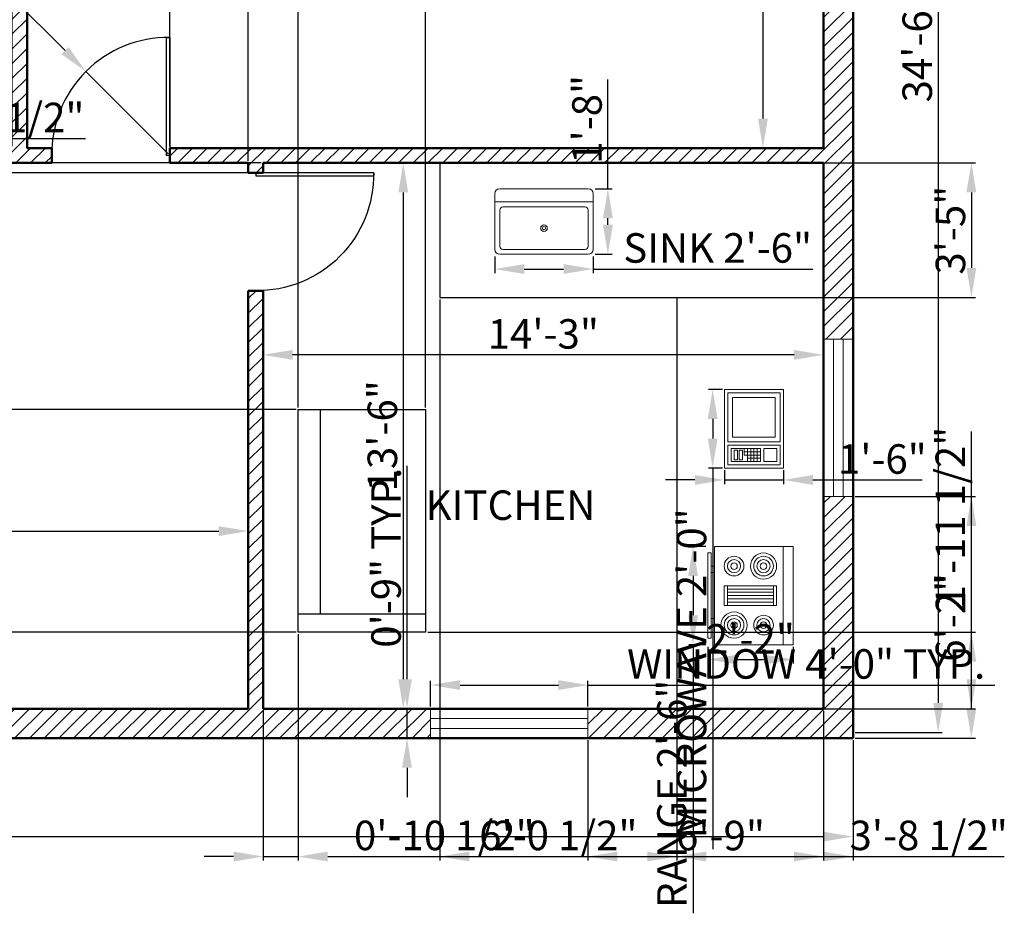
# Model space of a CAD drawing. Units: inches. Extents: x 61993 to 62774, y 55335 to 55871.
# Tile 5 of 6: x 62474 to 62774, y 55343 to 55615. Entities that reach past the tile are written whole.
import ezdxf

# ---------------------------------------------------------------- set-up
doc = ezdxf.new("R2010")
doc.units = ezdxf.units.IN
for name, color, linetype, lineweight in [('A-ANNO-DIMS', 2, 'Continuous', 18), ('A-AREA-IDEN', 7, 'Continuous', 25), ('A-DOOR', 3, 'Continuous', 25), ('A-EQPM', 8, 'Continuous', 18), ('A-FLOR-CASE', 9, 'Continuous', 25), ('A-FLOR-FIXT', 9, 'Continuous', 18), ('A-GLAZ', 4, 'Continuous', 18), ('A-WALL', 7, 'Continuous', 50)]:
    doc.layers.add(name, color=color, linetype=linetype, lineweight=lineweight)
doc.layers.add('A-WALL-PATT', color=40, linetype='Continuous', lineweight=13, true_color=0xf8d731)
doc.styles.get("Standard").update_dxf_attribs({"font": 'arial.ttf'})
doc.dimstyles.new('ISO-25', dxfattribs={"dimtxt": 9, "dimasz": 9, "dimexe": 1.25, "dimexo": 0.625, "dimtad": 1, "dimdec": 1, "dimrnd": 9, "dimlunit": 3, "dimtxsty": 'Standard', "dimcen": 2.5, "dimadec": 0, "dimazin": 0, "dimtfac": 1, "dimtdec": 1, "dimtmove": 0, "dimatfit": 3, "dimfxl": 1, "dimarcsym": 0})

# ---------------------------------------------------------------- blocks, each defined once
blk = doc.blocks.new('*D7')
at = {"layer": 'A-ANNO-DIMS', "color": 0, "lineweight": -2, "transparency": 16777216}
for p, q in [((62718.57, 55806.96), (62699.45, 55806.96)), ((62700.7, 55797.96), (62700.7, 55584.96)), ((62718.57, 55575.96), (62699.45, 55575.96))]:
    blk.add_line(p, q, dxfattribs=at)
at = {"layer": 'A-ANNO-DIMS', "color": 0, "transparency": 16777216}
for points in [[(62699.2, 55797.96), (62702.2, 55797.96), (62700.7, 55806.96)], [(62699.2, 55584.96), (62702.2, 55584.96), (62700.7, 55575.96)]]:
    blk.add_solid(points, dxfattribs=at)
at = {"layer": 'Defpoints', "color": 0, "transparency": 16777216}
for p in [(62719.19, 55806.96), (62700.7, 55575.96), (62719.19, 55575.96)]:
    blk.add_point(p, dxfattribs=at)
at = {"layer": 'A-ANNO-DIMS', "color": 0, "transparency": 16777216, "insert": (62695.48, 55691.46), "char_height": 9, "attachment_point": 5, "rotation": 90}
blk.add_mtext('19\'-6"', dxfattribs=at)
blk = doc.blocks.new('*D9')
at = {"layer": 'A-ANNO-DIMS', "color": 0, "lineweight": -2, "transparency": 16777216}
for p, q in [((62718.57, 55571.46), (62589.72, 55571.46)), ((62590.97, 55562.46), (62590.97, 55413.96)), ((62718.57, 55404.96), (62589.72, 55404.96))]:
    blk.add_line(p, q, dxfattribs=at)
at = {"layer": 'A-ANNO-DIMS', "color": 0, "transparency": 16777216}
for points in [[(62589.47, 55562.46), (62592.47, 55562.46), (62590.97, 55571.46)], [(62589.47, 55413.96), (62592.47, 55413.96), (62590.97, 55404.96)]]:
    blk.add_solid(points, dxfattribs=at)
at = {"layer": 'Defpoints', "color": 0, "transparency": 16777216}
for p in [(62719.19, 55571.46), (62590.97, 55404.96), (62719.19, 55404.96)]:
    blk.add_point(p, dxfattribs=at)
at = {"layer": 'A-ANNO-DIMS', "color": 0, "transparency": 16777216, "insert": (62585.75, 55488.21), "char_height": 9, "attachment_point": 5, "rotation": 90}
blk.add_mtext('13\'-6"', dxfattribs=at)
blk = doc.blocks.new('*D10')
at = {"layer": 'A-ANNO-DIMS', "color": 0, "lineweight": -2, "transparency": 16777216}
for p, q in [((62548.19, 55405.58), (62548.19, 55514.14)), ((62710.19, 55512.89), (62557.19, 55512.89)), ((62719.19, 55405.58), (62719.19, 55514.14))]:
    blk.add_line(p, q, dxfattribs=at)
at = {"layer": 'A-ANNO-DIMS', "color": 0, "transparency": 16777216}
for points in [[(62557.19, 55514.39), (62557.19, 55511.39), (62548.19, 55512.89)], [(62710.19, 55514.39), (62710.19, 55511.39), (62719.19, 55512.89)]]:
    blk.add_solid(points, dxfattribs=at)
at = {"layer": 'Defpoints', "color": 0, "transparency": 16777216}
for p in [(62548.19, 55512.89), (62548.19, 55404.96), (62719.19, 55404.96)]:
    blk.add_point(p, dxfattribs=at)
at = {"layer": 'A-ANNO-DIMS', "color": 0, "transparency": 16777216, "insert": (62633.69, 55518.11), "char_height": 9, "attachment_point": 5}
blk.add_mtext('14\'-3"', dxfattribs=at)
blk = doc.blocks.new('*D12')
at = {"layer": 'A-ANNO-DIMS', "color": 0, "lineweight": -2, "transparency": 16777216}
for p, q in [((62077.82, 55405.58), (62077.82, 55460.37)), ((62086.82, 55459.12), (62534.69, 55459.12)), ((62543.69, 55405.58), (62543.69, 55460.37))]:
    blk.add_line(p, q, dxfattribs=at)
at = {"layer": 'A-ANNO-DIMS', "color": 0, "transparency": 16777216}
for points in [[(62086.82, 55460.62), (62086.82, 55457.62), (62077.82, 55459.12)], [(62534.69, 55460.62), (62534.69, 55457.62), (62543.69, 55459.12)]]:
    blk.add_solid(points, dxfattribs=at)
at = {"layer": 'Defpoints', "color": 0, "transparency": 16777216}
for p in [(62543.69, 55459.12), (62077.82, 55404.96), (62543.69, 55404.96)]:
    blk.add_point(p, dxfattribs=at)
at = {"layer": 'A-ANNO-DIMS', "color": 0, "transparency": 16777216, "insert": (62310.76, 55464.35), "char_height": 9, "attachment_point": 5}
blk.add_mtext("39'", dxfattribs=at)
blk = doc.blocks.new('Sink-single - 30 in top')
blk.add_line((-15, -3.999996), (15, -3.999996))
for points in [[(-13.5, 0), (13.5, 0)], [(-15, -18.499996), (-15, -1.5)], [(15, -1.5), (15, -18.499996)], [(-12.5, -5.499996), (12.5, -5.499996)], [(-13.5, -17.499996), (-13.5, -6.499996)], [(13.5, -6.499996), (13.5, -17.499996)], [(13.5, -19.999996), (-13.5, -19.999996)], [(12.5, -18.499996), (-12.5, -18.499996)]]:
    blk.add_lwpolyline(points)
for radius in [1, 0.5]:
    blk.add_circle((0, -11.999996), radius)
for centre, radius, start, end in [((-13.5, -1.5), 1.5, 90, 180), ((13.5, -1.5), 1.5, 0, 90), ((-12.5, -6.499996), 1, 90, 180), ((12.5, -6.499996), 1, 0, 90), ((-12.5, -17.499996), 1, 180, 270), ((12.5, -17.499996), 1, 270, 0), ((-13.5, -18.499996), 1.5, 180, 270), ((13.5, -18.499996), 1.5, 270, 0)]:
    blk.add_arc(centre, radius, start, end)
blk = doc.blocks.new('Range-Oven - 30 in top')
for p, q in [((0, -3), (30, -3)), ((12, -6), (18, -6)), ((13, -20), (13, -6)), ((14, -6), (14, -20)), ((15, -20), (15, -6)), ((16, -6), (16, -20)), ((17, -20), (17, -6)), ((18, -20), (12, -20)), ((6, -24), (6, -25)), ((8, -25), (8, -24)), ((22, -25), (22, -24)), ((24, -24), (24, -25))]:
    blk.add_line(p, q)
for points in [[(0, -24), (0, 0), (30, 0), (30, -24)], [(12, -21), (12, -5), (18, -5), (18, -21)], [(2, -26), (2, -25), (28, -25), (28, -26)]]:
    blk.add_lwpolyline(points, close=True)
for centre, radius in [((6, -9), 4), ((6, -9), 3), ((24, -9), 3), ((6, -9), 2), ((6, -9), 1), ((24, -9), 2), ((24, -9), 1), ((6, -18), 3), ((24, -18), 4), ((24, -18), 3), ((6, -18), 2), ((6, -18), 1), ((24, -18), 2), ((24, -18), 1)]:
    blk.add_circle(centre, radius)
blk = doc.blocks.new('Microwave')
for p, q in [((18, 10), (22, 10)), ((19, 7), (19, 11)), ((20, 11), (20, 7)), ((21, 7), (21, 11)), ((22, 9), (18, 9)), ((18, 8), (22, 8)), ((22, 7), (18, 7)), ((19, 6), (19, 7)), ((20, 7), (20, 6)), ((20, 6), (18, 6))]:
    blk.add_line(p, q)
for points in [[(0, 0), (0, 18), (24, 18), (24, 0)], [(1, 1), (1, 17), (16, 17), (16, 1)], [(2.5, 2.5), (2.5, 15.5), (14.5, 15.5), (14.5, 2.5)], [(17, 1), (17, 17), (23, 17), (23, 1)], [(18, 12), (18, 16), (22, 16), (22, 12)], [(18, 2), (18, 11), (22, 11), (22, 2)], [(18.5, 4.5), (18.5, 5.5), (21.5, 5.5), (21.5, 4.5)], [(18.5, 3), (18.5, 4), (21.5, 4), (21.5, 3)]]:
    blk.add_lwpolyline(points, close=True)
blk = doc.blocks.new('*D25')
at = {"layer": 'A-ANNO-DIMS', "color": 0, "lineweight": -2, "transparency": 16777216}
for p, q in [((62728.82, 55815.96), (62755.41, 55815.96)), ((62754.16, 55806.96), (62754.16, 55406.74)), ((62728.82, 55397.74), (62755.41, 55397.74))]:
    blk.add_line(p, q, dxfattribs=at)
at = {"layer": 'A-ANNO-DIMS', "color": 0, "transparency": 16777216}
for points in [[(62752.66, 55806.96), (62755.66, 55806.96), (62754.16, 55815.96)], [(62752.66, 55406.74), (62755.66, 55406.74), (62754.16, 55397.74)]]:
    blk.add_solid(points, dxfattribs=at)
at = {"layer": 'Defpoints', "color": 0, "transparency": 16777216}
for p in [(62728.19, 55815.96), (62728.19, 55397.74), (62754.16, 55397.74)]:
    blk.add_point(p, dxfattribs=at)
at = {"layer": 'A-ANNO-DIMS', "color": 0, "transparency": 16777216, "insert": (62748.93, 55606.85), "char_height": 9, "attachment_point": 5, "rotation": 90}
blk.add_mtext('34\'-6"', dxfattribs=at)
blk = doc.blocks.new('*D28')
at = {"layer": 'A-ANNO-DIMS', "color": 0, "lineweight": -2, "transparency": 16777216}
for p, q in [((62067.57, 55395.33), (62067.57, 55364.68)), ((62728.19, 55395.33), (62728.19, 55364.68)), ((62076.57, 55365.93), (62719.19, 55365.93))]:
    blk.add_line(p, q, dxfattribs=at)
at = {"layer": 'A-ANNO-DIMS', "color": 0, "transparency": 16777216}
for points in [[(62076.57, 55367.43), (62076.57, 55364.43), (62067.57, 55365.93)], [(62719.19, 55367.43), (62719.19, 55364.43), (62728.19, 55365.93)]]:
    blk.add_solid(points, dxfattribs=at)
at = {"layer": 'Defpoints', "color": 0, "transparency": 16777216}
for p in [(62067.57, 55395.96), (62728.19, 55395.96), (62728.19, 55365.93)]:
    blk.add_point(p, dxfattribs=at)
at = {"layer": 'A-ANNO-DIMS', "color": 0, "transparency": 16777216, "insert": (62397.88, 55371.15), "char_height": 9, "attachment_point": 5}
blk.add_mtext('54\'-9"', dxfattribs=at)
blk = doc.blocks.new('WIN-48IN')
for p, q in [((0, 9), (0, 0)), ((48, 9), (48, 0)), ((48, 6), (0, 6)), ((48, 3), (0, 3))]:
    blk.add_line(p, q)
blk = doc.blocks.new('DOOR-SINGLE-36IN')
for p, q in [((35, 0), (35, 36)), ((35, 36), (36, 36)), ((36, 36), (36, 2.25)), ((36, 0), (35, 0))]:
    blk.add_line(p, q)
blk.add_arc((35.5, 0.5), 35.5, 89.1931, 180.8069)
blk = doc.blocks.new('*D32')
at = {"layer": 'A-ANNO-DIMS', "color": 0, "lineweight": -2, "transparency": 16777216}
for p, q in [((62599.31, 55405.58), (62599.31, 55413.41)), ((62647.31, 55405.58), (62647.31, 55413.41)), ((62608.31, 55412.16), (62638.31, 55412.16)), ((62647.31, 55412.16), (62771.45, 55412.16))]:
    blk.add_line(p, q, dxfattribs=at)
at = {"layer": 'A-ANNO-DIMS', "color": 0, "transparency": 16777216}
for points in [[(62608.31, 55413.66), (62608.31, 55410.66), (62599.31, 55412.16)], [(62638.31, 55413.66), (62638.31, 55410.66), (62647.31, 55412.16)]]:
    blk.add_solid(points, dxfattribs=at)
at = {"layer": 'Defpoints', "color": 0, "transparency": 16777216}
for p in [(62647.31, 55412.16), (62599.31, 55404.96), (62647.31, 55404.96)]:
    blk.add_point(p, dxfattribs=at)
at = {"layer": 'A-ANNO-DIMS', "color": 0, "transparency": 16777216, "insert": (62713.88, 55417.44), "char_height": 9, "attachment_point": 5}
blk.add_mtext('WINDOW 4\'-0" TYP.', dxfattribs=at)
blk = doc.blocks.new('*D33')
at = {"layer": 'A-ANNO-DIMS', "color": 0, "lineweight": -2, "transparency": 16777216}
for p, q in [((62592.11, 55413.96), (62592.11, 55479.07)), ((62598.68, 55404.96), (62590.86, 55404.96)), ((62592.11, 55395.96), (62592.11, 55404.96)), ((62598.68, 55395.96), (62590.86, 55395.96)), ((62592.11, 55386.96), (62592.11, 55377.96))]:
    blk.add_line(p, q, dxfattribs=at)
at = {"layer": 'A-ANNO-DIMS', "color": 0, "transparency": 16777216}
for points in [[(62590.61, 55413.96), (62593.61, 55413.96), (62592.11, 55404.96)], [(62590.61, 55386.96), (62593.61, 55386.96), (62592.11, 55395.96)]]:
    blk.add_solid(points, dxfattribs=at)
at = {"layer": 'Defpoints', "color": 0, "transparency": 16777216}
for p in [(62592.11, 55404.96), (62599.31, 55404.96), (62599.31, 55395.96)]:
    blk.add_point(p, dxfattribs=at)
at = {"layer": 'A-ANNO-DIMS', "color": 0, "transparency": 16777216, "insert": (62586.89, 55451.01), "char_height": 9, "attachment_point": 5, "rotation": 90}
blk.add_mtext('0\'-9" TYP.', dxfattribs=at)
blk = doc.blocks.new('*D46')
at = {"layer": 'A-ANNO-DIMS', "color": 0, "lineweight": -2, "transparency": 16777216}
for p, q in [((62373.49, 55581.91), (62373.49, 55577.6)), ((62398.04, 55581.91), (62398.04, 55577.6)), ((62382.49, 55578.85), (62389.04, 55578.85)), ((62398.04, 55578.85), (62494.01, 55578.85))]:
    blk.add_line(p, q, dxfattribs=at)
at = {"layer": 'A-ANNO-DIMS', "color": 0, "transparency": 16777216}
for points in [[(62382.49, 55580.35), (62382.49, 55577.35), (62373.49, 55578.85)], [(62389.04, 55580.35), (62389.04, 55577.35), (62398.04, 55578.85)]]:
    blk.add_solid(points, dxfattribs=at)
at = {"layer": 'Defpoints', "color": 0, "transparency": 16777216}
for p in [(62373.49, 55582.54), (62398.04, 55582.54), (62398.04, 55578.85)]:
    blk.add_point(p, dxfattribs=at)
at = {"layer": 'A-ANNO-DIMS', "color": 0, "transparency": 16777216, "insert": (62450.52, 55584.13), "char_height": 9, "attachment_point": 5}
blk.add_mtext('BASIN 2\'-0 1/2"', dxfattribs=at)
blk = doc.blocks.new('*D50')
at = {"layer": 'A-ANNO-DIMS', "color": 0, "lineweight": -2, "transparency": 16777216}
for p, q in [((62618.9, 55542.93), (62618.9, 55537.81)), ((62648.9, 55542.93), (62648.9, 55537.81)), ((62627.9, 55539.06), (62639.9, 55539.06)), ((62648.9, 55539.06), (62715.87, 55539.06))]:
    blk.add_line(p, q, dxfattribs=at)
at = {"layer": 'A-ANNO-DIMS', "color": 0, "transparency": 16777216}
for points in [[(62627.9, 55540.56), (62627.9, 55537.56), (62618.9, 55539.06)], [(62639.9, 55540.56), (62639.9, 55537.56), (62648.9, 55539.06)]]:
    blk.add_solid(points, dxfattribs=at)
at = {"layer": 'Defpoints', "color": 0, "transparency": 16777216}
for p in [(62618.9, 55543.56), (62648.9, 55543.56), (62648.9, 55539.06)]:
    blk.add_point(p, dxfattribs=at)
at = {"layer": 'A-ANNO-DIMS', "color": 0, "transparency": 16777216, "insert": (62686.89, 55544.33), "char_height": 9, "attachment_point": 5}
blk.add_mtext('SINK 2\'-6"', dxfattribs=at)
blk = doc.blocks.new('*D51')
at = {"layer": 'A-ANNO-DIMS', "color": 0, "lineweight": -2, "transparency": 16777216}
for p, q in [((62653.4, 55563.56), (62653.4, 55596.88)), ((62649.53, 55563.56), (62654.65, 55563.56)), ((62653.4, 55552.56), (62653.4, 55554.56)), ((62649.53, 55543.56), (62654.65, 55543.56))]:
    blk.add_line(p, q, dxfattribs=at)
at = {"layer": 'A-ANNO-DIMS', "color": 0, "transparency": 16777216}
for points in [[(62651.9, 55554.56), (62654.9, 55554.56), (62653.4, 55563.56)], [(62651.9, 55552.56), (62654.9, 55552.56), (62653.4, 55543.56)]]:
    blk.add_solid(points, dxfattribs=at)
at = {"layer": 'Defpoints', "color": 0, "transparency": 16777216}
for p in [(62648.9, 55563.56), (62653.4, 55563.56), (62648.9, 55543.56)]:
    blk.add_point(p, dxfattribs=at)
at = {"layer": 'A-ANNO-DIMS', "color": 0, "transparency": 16777216, "insert": (62648.18, 55584.72), "char_height": 9, "attachment_point": 5, "rotation": 90}
blk.add_mtext('1\'-8"', dxfattribs=at)
blk = doc.blocks.new('*D52')
at = {"layer": 'A-ANNO-DIMS', "color": 0, "lineweight": -2, "transparency": 16777216}
for p, q in [((62683.26, 55454.45), (62678.13, 55454.45)), ((62679.38, 55445.45), (62679.38, 55433.45)), ((62683.26, 55424.45), (62678.13, 55424.45)), ((62679.38, 55424.45), (62679.38, 55342.54))]:
    blk.add_line(p, q, dxfattribs=at)
at = {"layer": 'A-ANNO-DIMS', "color": 0, "transparency": 16777216}
for points in [[(62677.88, 55445.45), (62680.88, 55445.45), (62679.38, 55454.45)], [(62677.88, 55433.45), (62680.88, 55433.45), (62679.38, 55424.45)]]:
    blk.add_solid(points, dxfattribs=at)
at = {"layer": 'Defpoints', "color": 0, "transparency": 16777216}
for p in [(62683.88, 55454.45), (62679.38, 55424.45), (62683.88, 55424.45)]:
    blk.add_point(p, dxfattribs=at)
at = {"layer": 'A-ANNO-DIMS', "color": 0, "transparency": 16777216, "insert": (62674.1, 55379), "char_height": 9, "attachment_point": 5, "rotation": 90}
blk.add_mtext('RANGE 2\'-6"', dxfattribs=at)
blk = doc.blocks.new('*D53')
at = {"layer": 'A-ANNO-DIMS', "color": 0, "lineweight": -2, "transparency": 16777216}
for p, q in [((62683.88, 55423.83), (62683.88, 55418.7)), ((62709.88, 55423.83), (62709.88, 55418.7)), ((62692.88, 55419.95), (62700.88, 55419.95))]:
    blk.add_line(p, q, dxfattribs=at)
at = {"layer": 'A-ANNO-DIMS', "color": 0, "transparency": 16777216}
for points in [[(62692.88, 55421.45), (62692.88, 55418.45), (62683.88, 55419.95)], [(62700.88, 55421.45), (62700.88, 55418.45), (62709.88, 55419.95)]]:
    blk.add_solid(points, dxfattribs=at)
at = {"layer": 'Defpoints', "color": 0, "transparency": 16777216}
for p in [(62683.88, 55424.45), (62709.88, 55424.45), (62709.88, 55419.95)]:
    blk.add_point(p, dxfattribs=at)
at = {"layer": 'A-ANNO-DIMS', "color": 0, "transparency": 16777216, "insert": (62696.88, 55425.1), "char_height": 9, "attachment_point": 5}
blk.add_mtext('2\'-2"', dxfattribs=at)
blk = doc.blocks.new('*D58')
at = {"layer": 'A-ANNO-DIMS', "color": 0, "lineweight": -2, "transparency": 16777216}
for p, q in [((62688.34, 55502.33), (62684.11, 55502.33)), ((62685.36, 55493.33), (62685.36, 55487.33)), ((62688.34, 55478.33), (62684.11, 55478.33)), ((62685.36, 55478.33), (62685.36, 55362.14))]:
    blk.add_line(p, q, dxfattribs=at)
at = {"layer": 'A-ANNO-DIMS', "color": 0, "transparency": 16777216}
for points in [[(62683.86, 55493.33), (62686.86, 55493.33), (62685.36, 55502.33)], [(62683.86, 55487.33), (62686.86, 55487.33), (62685.36, 55478.33)]]:
    blk.add_solid(points, dxfattribs=at)
at = {"layer": 'Defpoints', "color": 0, "transparency": 16777216}
for p in [(62688.96, 55502.33), (62685.36, 55478.33), (62688.96, 55478.33)]:
    blk.add_point(p, dxfattribs=at)
at = {"layer": 'A-ANNO-DIMS', "color": 0, "transparency": 16777216, "insert": (62680.08, 55415.74), "char_height": 9, "attachment_point": 5, "rotation": 90}
blk.add_mtext('MICROWAVE 2\'-0"', dxfattribs=at)
blk = doc.blocks.new('*D59')
at = {"layer": 'A-ANNO-DIMS', "color": 0, "lineweight": -2, "transparency": 16777216}
for p, q in [((62688.96, 55477.7), (62688.96, 55473.48)), ((62706.96, 55477.7), (62706.96, 55473.48)), ((62679.96, 55474.73), (62670.96, 55474.73)), ((62688.96, 55474.73), (62706.96, 55474.73)), ((62715.96, 55474.73), (62749.29, 55474.73))]:
    blk.add_line(p, q, dxfattribs=at)
at = {"layer": 'A-ANNO-DIMS', "color": 0, "transparency": 16777216}
for points in [[(62679.96, 55476.23), (62679.96, 55473.23), (62688.96, 55474.73)], [(62715.96, 55476.23), (62715.96, 55473.23), (62706.96, 55474.73)]]:
    blk.add_solid(points, dxfattribs=at)
at = {"layer": 'Defpoints', "color": 0, "transparency": 16777216}
for p in [(62688.96, 55478.33), (62706.96, 55478.33), (62706.96, 55474.73)]:
    blk.add_point(p, dxfattribs=at)
at = {"layer": 'A-ANNO-DIMS', "color": 0, "transparency": 16777216, "insert": (62737.13, 55479.95), "char_height": 9, "attachment_point": 5}
blk.add_mtext('1\'-6"', dxfattribs=at)
blk = doc.blocks.new('*D63')
at = {"layer": 'A-ANNO-DIMS', "color": 0, "lineweight": -2, "transparency": 16777216}
for p, q in [((62647.31, 55395.33), (62647.31, 55358.61)), ((62728.19, 55395.33), (62728.19, 55358.61)), ((62656.31, 55359.86), (62719.19, 55359.86))]:
    blk.add_line(p, q, dxfattribs=at)
at = {"layer": 'A-ANNO-DIMS', "color": 0, "transparency": 16777216}
for points in [[(62656.31, 55361.36), (62656.31, 55358.36), (62647.31, 55359.86)], [(62719.19, 55361.36), (62719.19, 55358.36), (62728.19, 55359.86)]]:
    blk.add_solid(points, dxfattribs=at)
at = {"layer": 'Defpoints', "color": 0, "transparency": 16777216}
for p in [(62647.31, 55395.96), (62728.19, 55395.96), (62728.19, 55359.86)]:
    blk.add_point(p, dxfattribs=at)
at = {"layer": 'A-ANNO-DIMS', "color": 0, "transparency": 16777216, "insert": (62687.75, 55365.08), "char_height": 9, "attachment_point": 5}
blk.add_mtext('6\'-9"', dxfattribs=at)
blk = doc.blocks.new('*D70')
at = {"layer": 'A-ANNO-DIMS', "color": 0, "lineweight": -2, "transparency": 16777216}
for p, q in [((62728.82, 55469.72), (62765.54, 55469.72)), ((62764.29, 55404.96), (62764.29, 55460.72)), ((62728.82, 55395.96), (62765.54, 55395.96))]:
    blk.add_line(p, q, dxfattribs=at)
at = {"layer": 'A-ANNO-DIMS', "color": 0, "transparency": 16777216}
for points in [[(62762.79, 55460.72), (62765.79, 55460.72), (62764.29, 55469.72)], [(62762.79, 55404.96), (62765.79, 55404.96), (62764.29, 55395.96)]]:
    blk.add_solid(points, dxfattribs=at)
at = {"layer": 'Defpoints', "color": 0, "transparency": 16777216}
for p in [(62728.19, 55469.72), (62764.29, 55469.72), (62728.19, 55395.96)]:
    blk.add_point(p, dxfattribs=at)
at = {"layer": 'A-ANNO-DIMS', "color": 0, "transparency": 16777216, "insert": (62759.07, 55432.84), "char_height": 9, "attachment_point": 5, "rotation": 90}
blk.add_mtext('6\'-2"', dxfattribs=at)
blk = doc.blocks.new('*D72')
at = {"layer": 'A-ANNO-DIMS', "color": 0, "lineweight": -2, "transparency": 16777216}
for p, q in [((62451.32, 55576.58), (62451.32, 55853.31)), ((62460.32, 55852.06), (62462.69, 55852.06)), ((62471.69, 55576.58), (62471.69, 55853.31)), ((62471.69, 55852.06), (62525.99, 55852.06))]:
    blk.add_line(p, q, dxfattribs=at)
at = {"layer": 'A-ANNO-DIMS', "color": 0, "transparency": 16777216}
for points in [[(62460.32, 55853.56), (62460.32, 55850.56), (62451.32, 55852.06)], [(62462.69, 55853.56), (62462.69, 55850.56), (62471.69, 55852.06)]]:
    blk.add_solid(points, dxfattribs=at)
at = {"layer": 'Defpoints', "color": 0, "transparency": 16777216}
for p in [(62471.69, 55852.06), (62451.32, 55575.96), (62471.69, 55575.96)]:
    blk.add_point(p, dxfattribs=at)
at = {"layer": 'A-ANNO-DIMS', "color": 0, "transparency": 16777216, "insert": (62503.34, 55857.33), "char_height": 9, "attachment_point": 5}
blk.add_mtext('1\'-8 1/2"', dxfattribs=at)
blk = doc.blocks.new('*D73')
at = {"layer": 'A-ANNO-DIMS', "color": 0, "lineweight": -2, "transparency": 16777216}
for p, q in [((62519.74, 55576.58), (62519.74, 55853.31)), ((62528.74, 55852.06), (62534.69, 55852.06)), ((62543.69, 55572.08), (62543.69, 55853.31)), ((62543.69, 55852.06), (62578.02, 55852.06))]:
    blk.add_line(p, q, dxfattribs=at)
at = {"layer": 'A-ANNO-DIMS', "color": 0, "transparency": 16777216}
for points in [[(62528.74, 55853.56), (62528.74, 55850.56), (62519.74, 55852.06)], [(62534.69, 55853.56), (62534.69, 55850.56), (62543.69, 55852.06)]]:
    blk.add_solid(points, dxfattribs=at)
at = {"layer": 'Defpoints', "color": 0, "transparency": 16777216}
for p in [(62543.69, 55852.06), (62519.74, 55575.96), (62543.69, 55571.46)]:
    blk.add_point(p, dxfattribs=at)
at = {"layer": 'A-ANNO-DIMS', "color": 0, "transparency": 16777216, "insert": (62565.36, 55857.28), "char_height": 9, "attachment_point": 5}
blk.add_mtext('2\'-0"', dxfattribs=at)
blk = doc.blocks.new('*D74')
at = {"layer": 'A-ANNO-DIMS', "color": 0, "lineweight": -2, "transparency": 16777216}
for p, q in [((62032.09, 55580.46), (62032.09, 55589.46)), ((62547.57, 55571.46), (62030.84, 55571.46)), ((62032.09, 55571.46), (62032.09, 55568.46)), ((62547.57, 55568.46), (62030.84, 55568.46)), ((62032.09, 55559.46), (62032.09, 55525.28))]:
    blk.add_line(p, q, dxfattribs=at)
at = {"layer": 'A-ANNO-DIMS', "color": 0, "transparency": 16777216}
for points in [[(62030.59, 55580.46), (62033.59, 55580.46), (62032.09, 55571.46)], [(62030.59, 55559.46), (62033.59, 55559.46), (62032.09, 55568.46)]]:
    blk.add_solid(points, dxfattribs=at)
at = {"layer": 'Defpoints', "color": 0, "transparency": 16777216}
for p in [(62548.19, 55571.46), (62032.09, 55568.46), (62548.19, 55568.46)]:
    blk.add_point(p, dxfattribs=at)
at = {"layer": 'A-ANNO-DIMS', "color": 0, "transparency": 16777216, "insert": (62026.87, 55537.87), "char_height": 9, "attachment_point": 5, "rotation": 90}
blk.add_mtext('0\'-3"', dxfattribs=at)
blk = doc.blocks.new('*D76')
at = {"layer": 'A-ANNO-DIMS', "color": 0, "lineweight": -2, "transparency": 16777216}
for p, q in [((62674.46, 55404.33), (62674.46, 55358.61)), ((62719.19, 55404.33), (62719.19, 55358.61)), ((62683.46, 55359.86), (62710.19, 55359.86)), ((62719.19, 55359.86), (62774.33, 55359.86))]:
    blk.add_line(p, q, dxfattribs=at)
at = {"layer": 'A-ANNO-DIMS', "color": 0, "transparency": 16777216}
for points in [[(62683.46, 55361.36), (62683.46, 55358.36), (62674.46, 55359.86)], [(62710.19, 55361.36), (62710.19, 55358.36), (62719.19, 55359.86)]]:
    blk.add_solid(points, dxfattribs=at)
at = {"layer": 'Defpoints', "color": 0, "transparency": 16777216}
for p in [(62674.46, 55404.96), (62719.19, 55404.96), (62719.19, 55359.86)]:
    blk.add_point(p, dxfattribs=at)
at = {"layer": 'A-ANNO-DIMS', "color": 0, "transparency": 16777216, "insert": (62751.26, 55365.14), "char_height": 9, "attachment_point": 5}
blk.add_mtext('3\'-8 1/2"', dxfattribs=at)
blk = doc.blocks.new('*D77')
at = {"layer": 'A-ANNO-DIMS', "color": 0, "lineweight": -2, "transparency": 16777216}
for p, q in [((62602.74, 55571.46), (62765.54, 55571.46)), ((62764.29, 55562.46), (62764.29, 55539.41)), ((62602.74, 55530.41), (62765.54, 55530.41))]:
    blk.add_line(p, q, dxfattribs=at)
at = {"layer": 'A-ANNO-DIMS', "color": 0, "transparency": 16777216}
for points in [[(62762.79, 55562.46), (62765.79, 55562.46), (62764.29, 55571.46)], [(62762.79, 55539.41), (62765.79, 55539.41), (62764.29, 55530.41)]]:
    blk.add_solid(points, dxfattribs=at)
at = {"layer": 'Defpoints', "color": 0, "transparency": 16777216}
for p in [(62602.11, 55571.46), (62602.11, 55530.41), (62764.29, 55530.41)]:
    blk.add_point(p, dxfattribs=at)
at = {"layer": 'A-ANNO-DIMS', "color": 0, "transparency": 16777216, "insert": (62759.07, 55550.93), "char_height": 9, "attachment_point": 5, "rotation": 90}
blk.add_mtext('3\'-5"', dxfattribs=at)
blk = doc.blocks.new('*D78')
at = {"layer": 'A-ANNO-DIMS', "color": 0, "lineweight": -2, "transparency": 16777216}
for p, q in [((62602.11, 55529.79), (62602.11, 55358.61)), ((62674.46, 55529.79), (62674.46, 55358.61)), ((62611.11, 55359.86), (62665.46, 55359.86))]:
    blk.add_line(p, q, dxfattribs=at)
at = {"layer": 'A-ANNO-DIMS', "color": 0, "transparency": 16777216}
for points in [[(62611.11, 55361.36), (62611.11, 55358.36), (62602.11, 55359.86)], [(62665.46, 55361.36), (62665.46, 55358.36), (62674.46, 55359.86)]]:
    blk.add_solid(points, dxfattribs=at)
at = {"layer": 'Defpoints', "color": 0, "transparency": 16777216}
for p in [(62602.11, 55530.41), (62674.46, 55530.41), (62674.46, 55359.86)]:
    blk.add_point(p, dxfattribs=at)
at = {"layer": 'A-ANNO-DIMS', "color": 0, "transparency": 16777216, "insert": (62638.28, 55365.13), "char_height": 9, "attachment_point": 5}
blk.add_mtext('6\'-0 1/2"', dxfattribs=at)
blk = doc.blocks.new('*D79')
at = {"layer": 'A-ANNO-DIMS', "color": 0, "lineweight": -2, "transparency": 16777216}
for p, q in [((62558.91, 55496.8), (62558.91, 55853.31)), ((62567.91, 55852.06), (62588.8, 55852.06)), ((62597.8, 55496.8), (62597.8, 55853.31))]:
    blk.add_line(p, q, dxfattribs=at)
at = {"layer": 'A-ANNO-DIMS', "color": 0, "transparency": 16777216}
for points in [[(62567.91, 55853.56), (62567.91, 55850.56), (62558.91, 55852.06)], [(62588.8, 55853.56), (62588.8, 55850.56), (62597.8, 55852.06)]]:
    blk.add_solid(points, dxfattribs=at)
at = {"layer": 'Defpoints', "color": 0, "transparency": 16777216}
for p in [(62597.8, 55852.06), (62558.91, 55496.17), (62597.8, 55496.17)]:
    blk.add_point(p, dxfattribs=at)
at = {"layer": 'A-ANNO-DIMS', "color": 0, "transparency": 16777216, "insert": (62578.36, 55857.28), "char_height": 9, "attachment_point": 5}
blk.add_mtext('3\'-3"', dxfattribs=at)
blk = doc.blocks.new('*D80')
at = {"layer": 'A-ANNO-DIMS', "color": 0, "lineweight": -2, "transparency": 16777216}
for p, q in [((62558.29, 55496.17), (62030.84, 55496.17)), ((62032.09, 55437.26), (62032.09, 55487.17)), ((62558.29, 55428.26), (62030.84, 55428.26))]:
    blk.add_line(p, q, dxfattribs=at)
at = {"layer": 'A-ANNO-DIMS', "color": 0, "transparency": 16777216}
for points in [[(62030.59, 55487.17), (62033.59, 55487.17), (62032.09, 55496.17)], [(62030.59, 55437.26), (62033.59, 55437.26), (62032.09, 55428.26)]]:
    blk.add_solid(points, dxfattribs=at)
at = {"layer": 'Defpoints', "color": 0, "transparency": 16777216}
for p in [(62032.09, 55496.17), (62558.91, 55496.17), (62558.91, 55428.26)]:
    blk.add_point(p, dxfattribs=at)
at = {"layer": 'A-ANNO-DIMS', "color": 0, "transparency": 16777216, "insert": (62026.87, 55462.22), "char_height": 9, "attachment_point": 5, "rotation": 90}
blk.add_mtext('5\'-8"', dxfattribs=at)
blk = doc.blocks.new('*D81')
at = {"layer": 'A-ANNO-DIMS', "color": 0, "lineweight": -2, "transparency": 16777216}
for p, q in [((62558.91, 55427.64), (62558.91, 55358.61)), ((62548.19, 55404.33), (62548.19, 55358.61)), ((62539.19, 55359.86), (62530.19, 55359.86)), ((62548.19, 55359.86), (62558.91, 55359.86)), ((62567.91, 55359.86), (62630.05, 55359.86))]:
    blk.add_line(p, q, dxfattribs=at)
at = {"layer": 'A-ANNO-DIMS', "color": 0, "transparency": 16777216}
for points in [[(62539.19, 55361.36), (62539.19, 55358.36), (62548.19, 55359.86)], [(62567.91, 55361.36), (62567.91, 55358.36), (62558.91, 55359.86)]]:
    blk.add_solid(points, dxfattribs=at)
at = {"layer": 'Defpoints', "color": 0, "transparency": 16777216}
for p in [(62558.91, 55428.26), (62548.19, 55404.96), (62558.91, 55359.86)]:
    blk.add_point(p, dxfattribs=at)
at = {"layer": 'A-ANNO-DIMS', "color": 0, "transparency": 16777216, "insert": (62603.48, 55365.13), "char_height": 9, "attachment_point": 5}
blk.add_mtext('0\'-10 1/2"', dxfattribs=at)
blk = doc.blocks.new('*D82')
at = {"layer": 'A-ANNO-DIMS', "color": 0, "lineweight": -2, "transparency": 16777216}
for p, q in [((62764.29, 55428.26), (62764.29, 55489.55)), ((62598.43, 55428.26), (62765.54, 55428.26)), ((62764.29, 55413.96), (62764.29, 55419.26)), ((62599.93, 55404.96), (62765.54, 55404.96))]:
    blk.add_line(p, q, dxfattribs=at)
at = {"layer": 'A-ANNO-DIMS', "color": 0, "transparency": 16777216}
for points in [[(62762.79, 55419.26), (62765.79, 55419.26), (62764.29, 55428.26)], [(62762.79, 55413.96), (62765.79, 55413.96), (62764.29, 55404.96)]]:
    blk.add_solid(points, dxfattribs=at)
at = {"layer": 'Defpoints', "color": 0, "transparency": 16777216}
for p in [(62597.8, 55428.26), (62764.29, 55428.26), (62599.31, 55404.96)]:
    blk.add_point(p, dxfattribs=at)
at = {"layer": 'A-ANNO-DIMS', "color": 0, "transparency": 16777216, "insert": (62759.02, 55463.41), "char_height": 9, "attachment_point": 5, "rotation": 90}
blk.add_mtext('1\'-11 1/2"', dxfattribs=at)
blk = doc.blocks.new('*D87')
at = {"layer": 'A-ANNO-DIMS', "color": 0, "lineweight": -2, "transparency": 16777216}
for p, q in [((62424.07, 55669.37), (62487.77, 55605.68)), ((62519.24, 55574.21), (62494.13, 55599.31))]:
    blk.add_line(p, q, dxfattribs=at)
at = {"layer": 'A-ANNO-DIMS', "color": 0, "transparency": 16777216}
blk.add_solid([(62488.83, 55606.74), (62486.71, 55604.61), (62494.13, 55599.31)], dxfattribs=at)
at = {"layer": 'Defpoints', "color": 0, "transparency": 16777216}
for p in [(62494.13, 55599.31), (62519.24, 55574.21)]:
    blk.add_point(p, dxfattribs=at)
at = {"layer": 'A-ANNO-DIMS', "color": 0, "transparency": 16777216, "insert": (62456.47, 55644.44), "char_height": 9, "attachment_point": 5, "rotation": 315}
blk.add_mtext('3X R2\'-11 1/2"', dxfattribs=at)

msp = doc.modelspace()

# ---------------------------------------------------------------- hatches: boundary and pattern name
at = {"layer": 'A-WALL-PATT'}
h = msp.add_hatch(dxfattribs=at)
h.set_pattern_fill('ANSI31', color=256)
h.paths.add_polyline_path([(62077.19, 55665.16), (62068.19, 55665.16), (62068.19, 55518.96), (62077.19, 55518.96), (62077.19, 55571.46), (62234.23, 55571.46), (62234.23, 55573.71, -0.007042), (62234.23, 55574.71), (62234.23, 55575.96), (62077.19, 55575.96)])
h.paths.add_polyline_path([(62077.19, 55806.96), (62138.51, 55806.96), (62138.51, 55815.96), (62068.19, 55815.96), (62068.19, 55713.16), (62077.19, 55713.16)])
h.paths.add_polyline_path([(62364.31, 55815.96), (62186.51, 55815.96), (62186.51, 55806.96), (62308.19, 55806.96), (62308.19, 55575.96), (62270.23, 55575.96), (62270.23, 55571.46), (62415.32, 55571.46), (62415.32, 55573.71, -0.007042), (62415.32, 55574.71), (62415.32, 55575.96), (62312.69, 55575.96), (62312.69, 55739.46), (62471.69, 55739.46), (62471.69, 55575.96), (62451.32, 55575.96), (62451.32, 55571.46), (62483.74, 55571.46), (62483.74, 55573.71, -0.007042), (62483.74, 55574.71), (62483.74, 55575.96), (62476.19, 55575.96), (62476.19, 55806.96), (62578.07, 55806.96), (62578.07, 55815.96), (62412.31, 55815.96), (62412.31, 55806.96), (62471.69, 55806.96), (62471.69, 55743.96), (62312.69, 55743.96), (62312.69, 55806.96), (62364.31, 55806.96)])
h.paths.add_polyline_path([(62728.19, 55815.96), (62626.07, 55815.96), (62626.07, 55806.96), (62719.19, 55806.96), (62719.19, 55739.46), (62728.19, 55739.46)])
h.paths.add_polyline_path([(62728.19, 55691.46), (62719.19, 55691.46), (62719.19, 55575.96), (62519.74, 55575.96), (62519.74, 55571.46), (62543.69, 55571.46), (62543.69, 55568.46), (62548.19, 55568.46), (62548.19, 55571.46), (62719.19, 55571.46), (62719.19, 55517.72), (62728.19, 55517.72)])
h.paths.add_polyline_path([(62599.31, 55404.96), (62548.19, 55404.96), (62548.19, 55532.46), (62546.94, 55532.46, -0.007042), (62545.94, 55532.46), (62543.69, 55532.46), (62543.69, 55404.96), (62444.22, 55404.96), (62444.22, 55395.96), (62599.31, 55395.96)])
h.paths.add_polyline_path([(62728.19, 55469.72), (62719.19, 55469.72), (62719.19, 55404.96), (62647.31, 55404.96), (62647.31, 55395.96), (62728.19, 55395.96)])
h.paths.add_polyline_path([(62396.22, 55404.96), (62309.17, 55404.96), (62309.17, 55395.96), (62396.22, 55395.96)])
h.paths.add_polyline_path([(62213.17, 55404.96), (62077.19, 55404.96), (62077.19, 55470.96), (62068.19, 55470.96), (62068.19, 55395.96), (62213.17, 55395.96)])

# ---------------------------------------------------------------- linework, layer by layer
at = {"layer": 'A-FLOR-CASE'}
for p, q in [((62602.11, 55571.46), (62602.11, 55530.41)), ((62602.11, 55530.41), (62674.46, 55530.41)), ((62674.46, 55530.41), (62674.46, 55404.96)), ((62565.64, 55496.17), (62565.64, 55433.94)), ((62558.91, 55433.94), (62597.8, 55433.94))]:
    msp.add_line(p, q, dxfattribs=at)
msp.add_lwpolyline([(62558.91, 55496.17), (62597.8, 55496.17), (62597.8, 55428.26), (62558.91, 55428.26)], close=True, dxfattribs=at)
at = {"layer": 'A-WALL'}
for p, q in [((62728.19, 55395.96), (62728.19, 55815.96)), ((62476.19, 55806.96), (62476.19, 55575.96)), ((62719.19, 55575.96), (62719.19, 55806.96)), ((62483.74, 55575.96), (62476.19, 55575.96)), ((62483.74, 55575.96), (62483.74, 55571.46)), ((62719.19, 55575.96), (62519.74, 55575.96)), ((62519.74, 55575.96), (62519.74, 55571.46)), ((62483.74, 55571.46), (62451.32, 55571.46)), ((62543.69, 55571.46), (62519.74, 55571.46)), ((62543.69, 55568.46), (62543.69, 55571.46)), ((62719.19, 55571.46), (62548.19, 55571.46)), ((62548.19, 55568.46), (62548.19, 55571.46)), ((62719.19, 55404.96), (62719.19, 55571.46)), ((62543.69, 55568.46), (62548.19, 55568.46)), ((62543.69, 55404.96), (62543.69, 55532.46)), ((62543.69, 55532.46), (62548.19, 55532.46)), ((62548.19, 55404.96), (62548.19, 55532.46)), ((62309.17, 55404.96), (62543.69, 55404.96)), ((62548.19, 55404.96), (62719.19, 55404.96)), ((62309.17, 55395.96), (62728.19, 55395.96))]:
    msp.add_line(p, q, dxfattribs=at)

# ---------------------------------------------------------------- block references
at = {"layer": 'A-DOOR'}
msp.add_blockref('DOOR-SINGLE-36IN', (62483.74, 55573.71), dxfattribs=at)
at = {"layer": 'A-DOOR', "extrusion": (0, 0, -1), "zscale": -1, "rotation": 90.00000000000497}
msp.add_blockref('DOOR-SINGLE-36IN', (-62545.94, 55532.45), dxfattribs=at)
at = {"layer": 'A-EQPM', "rotation": 270}
for name, p in [('Microwave', (62688.96, 55502.33)), ('Range-Oven - 30 in top', (62709.88, 55454.45))]:
    msp.add_blockref(name, p, dxfattribs=at)
at = {"layer": 'A-FLOR-FIXT'}
msp.add_blockref('Sink-single - 30 in top', (62633.9, 55563.56), dxfattribs=at)
at = {"layer": 'A-GLAZ', "rotation": 269.9999999999769}
msp.add_blockref('WIN-48IN', (62719.19, 55517.72), dxfattribs=at)
at = {"layer": 'A-GLAZ'}
msp.add_blockref('WIN-48IN', (62599.31, 55395.96), dxfattribs=at)

# ---------------------------------------------------------------- texts
at = {"layer": 'A-AREA-IDEN', "insert": (62597.8, 55471.53), "char_height": 9, "attachment_point": 1}
msp.add_mtext_dynamic_manual_height_columns('KITCHEN', width=116.6414, gutter_width=12.5, heights=[0], dxfattribs=at)

# ---------------------------------------------------------------- dimensions: what is measured, and where the dimension line sits
at = {"layer": 'A-ANNO-DIMS'}
for base, p1, p2, override, picture, middle in [((62471.69, 55852.06), (62451.32, 55575.96), (62471.69, 55575.96), {"dimdec": 1, "dimlfac": 1, "dimrnd": 0, "dimzin": 1, "dimdsep": 46, "dimlunit": 4, "dimfrac": 2}, '*D72', (62503.34, 55857.33)), ((62543.6945, 55852.0565), (62519.7385, 55575.9565), (62543.6945, 55571.4565), {"dimdec": 1, "dimlfac": 1, "dimrnd": 0, "dimzin": 1, "dimdsep": 46, "dimlunit": 4, "dimfrac": 2}, '*D73', (62565.3584, 55857.2767)), ((62597.8, 55852.06), (62558.91, 55496.17), (62597.8, 55496.17), {"dimdec": 1, "dimlfac": 1, "dimrnd": 0, "dimzin": 1, "dimdsep": 46, "dimlunit": 4, "dimfrac": 2}, '*D79', (62578.36, 55857.28)), ((62674.4592, 55359.8565), (62602.1103, 55530.4131), (62674.4592, 55530.4131), {"dimdec": 1, "dimlfac": 1, "dimrnd": 0, "dimzin": 1, "dimdsep": 46, "dimlunit": 4, "dimfrac": 2}, '*D78', (62638.2848, 55365.135)), ((62548.19, 55512.89), (62719.19, 55404.96), (62548.19, 55404.96), {"dimclrd": 0, "dimclre": 0, "dimclrt": 0}, '*D10', (62633.69, 55518.11)), ((62706.96, 55474.73), (62688.96, 55478.33), (62706.96, 55478.33), {"dimdec": 1, "dimlfac": 1, "dimrnd": 0, "dimzin": 1, "dimdsep": 46, "dimlunit": 4, "dimfrac": 2}, '*D59', (62737.13, 55479.95)), ((62543.69, 55459.12), (62077.82, 55404.96), (62543.69, 55404.96), {"dimclrd": 0, "dimclre": 0, "dimclrt": 0}, '*D12', (62310.76, 55464.35)), ((62709.88, 55419.95), (62683.88, 55424.45), (62709.88, 55424.45), {"dimdec": 1, "dimlfac": 1, "dimrnd": 0, "dimzin": 1, "dimdsep": 46, "dimlunit": 4, "dimfrac": 2}, '*D53', (62696.88, 55425.1)), ((62558.91, 55359.86), (62548.19, 55404.96), (62558.91, 55428.26), {"dimdec": 1, "dimlfac": 1, "dimrnd": 0, "dimzin": 1, "dimdsep": 46, "dimlunit": 4, "dimfrac": 2}, '*D81', (62603.48, 55365.13)), ((62719.19, 55359.86), (62674.46, 55404.96), (62719.19, 55404.96), {"dimdec": 1, "dimlfac": 1, "dimrnd": 0, "dimzin": 1, "dimdsep": 46, "dimlunit": 4, "dimfrac": 2}, '*D76', (62751.26, 55365.14)), ((62728.19, 55359.86), (62647.31, 55395.96), (62728.19, 55395.96), {"dimdec": 1, "dimlfac": 1, "dimrnd": 0, "dimzin": 1, "dimdsep": 46, "dimlunit": 4, "dimfrac": 2}, '*D63', (62687.75, 55365.08))]:
    dim = msp.add_linear_dim(base=base, p1=p1, p2=p2, dimstyle='ISO-25', override=override, dxfattribs=at)
    dim.commit()
    dim.dimension.update_dxf_attribs({"geometry": picture, "text_midpoint": middle})
for base, p1, p2, override, picture, middle in [((62754.16, 55397.74), (62728.19, 55815.96), (62728.19, 55397.74), {"dimclrd": 0, "dimclre": 0, "dimclrt": 0}, '*D25', (62748.93, 55606.85)), ((62700.7, 55575.96), (62719.19, 55806.96), (62719.19, 55575.96), {"dimclrd": 0, "dimclre": 0, "dimclrt": 0}, '*D7', (62695.48, 55691.46)), ((62653.4, 55563.56), (62648.9, 55543.56), (62648.9, 55563.56), {"dimdec": 1, "dimlfac": 1, "dimrnd": 0, "dimzin": 1, "dimdsep": 46, "dimlunit": 4, "dimfrac": 2}, '*D51', (62648.18, 55584.72)), ((62032.09, 55568.46), (62548.19, 55571.46), (62548.19, 55568.46), {"dimdec": 1, "dimlfac": 1, "dimrnd": 0, "dimzin": 1, "dimdsep": 46, "dimlunit": 4, "dimfrac": 2}, '*D74', (62026.87, 55537.87)), ((62590.97, 55404.96), (62719.19, 55571.46), (62719.19, 55404.96), {"dimclrd": 0, "dimclre": 0, "dimclrt": 0}, '*D9', (62585.75, 55488.21)), ((62764.2945, 55530.4131), (62602.1103, 55571.4565), (62602.1103, 55530.4131), {"dimdec": 1, "dimlfac": 1, "dimrnd": 0, "dimzin": 1, "dimdsep": 46, "dimlunit": 4, "dimfrac": 2}, '*D77', (62759.0713, 55550.9348)), ((62032.09, 55496.17), (62558.91, 55428.26), (62558.91, 55496.17), {"dimdec": 1, "dimlfac": 1, "dimrnd": 0, "dimzin": 1, "dimdsep": 46, "dimlunit": 4, "dimfrac": 2}, '*D80', (62026.87, 55462.22)), ((62764.29, 55428.26), (62599.31, 55404.96), (62597.8, 55428.26), {"dimdec": 1, "dimlfac": 1, "dimrnd": 0, "dimzin": 1, "dimdsep": 46, "dimlunit": 4, "dimfrac": 2}, '*D82', (62759.02, 55463.41)), ((62764.29, 55469.72), (62728.19, 55395.96), (62728.19, 55469.72), {"dimdec": 1, "dimlfac": 1, "dimrnd": 0, "dimzin": 1, "dimdsep": 46, "dimlunit": 4, "dimfrac": 2}, '*D70', (62759.07, 55432.84))]:
    dim = msp.add_linear_dim(base=base, p1=p1, p2=p2, angle=90, dimstyle='ISO-25', override=override, dxfattribs=at)
    dim.commit()
    dim.dimension.update_dxf_attribs({"geometry": picture, "text_midpoint": middle})
dim = msp.add_radius_dim(center=(62519.24, 55574.21), mpoint=(62494.13, 55599.31), text='3X <>', dimstyle='ISO-25', override={"dimdec": 1, "dimlfac": 1, "dimrnd": 0, "dimzin": 1, "dimdsep": 46, "dimlunit": 4, "dimfrac": 2}, dxfattribs=at)
dim.commit()
dim.dimension.update_dxf_attribs({"geometry": '*D87', "text_midpoint": (62456.47, 55644.44)})
for base, p1, p2, text, picture, middle in [((62398.0388, 55578.8531), (62373.4879, 55582.5357), (62398.0388, 55582.5357), 'BASIN <>', '*D46', (62450.5243, 55584.1315)), ((62648.9, 55539.06), (62618.9, 55543.56), (62648.9, 55543.56), 'SINK <>', '*D50', (62686.89, 55544.33)), ((62647.31, 55412.16), (62599.31, 55404.96), (62647.31, 55404.96), 'WINDOW <> TYP.', '*D32', (62713.88, 55417.44))]:
    dim = msp.add_linear_dim(base=base, p1=p1, p2=p2, text=text, dimstyle='ISO-25', override={"dimdec": 1, "dimlfac": 1, "dimrnd": 0, "dimzin": 1, "dimdsep": 46, "dimlunit": 4, "dimfrac": 2}, dxfattribs=at)
    dim.commit()
    dim.dimension.update_dxf_attribs({"geometry": picture, "text_midpoint": middle})
for base, p1, p2, angle, text, picture, middle in [((62685.36, 55478.33), (62688.96, 55502.33), (62688.96, 55478.33), 270, 'MICROWAVE <>', '*D58', (62680.08, 55415.74)), ((62592.11, 55404.96), (62599.31, 55395.96), (62599.31, 55404.96), 90, '<> TYP.', '*D33', (62586.89, 55451.01)), ((62679.38, 55424.45), (62683.88, 55454.45), (62683.88, 55424.45), 270, 'RANGE <>', '*D52', (62674.1, 55379))]:
    dim = msp.add_linear_dim(base=base, p1=p1, p2=p2, angle=angle, text=text, dimstyle='ISO-25', override={"dimdec": 1, "dimlfac": 1, "dimrnd": 0, "dimzin": 1, "dimdsep": 46, "dimlunit": 4, "dimfrac": 2}, dxfattribs=at)
    dim.commit()
    dim.dimension.update_dxf_attribs({"geometry": picture, "text_midpoint": middle})
dim = msp.add_aligned_dim(p1=(62067.57, 55395.96), p2=(62728.19, 55395.96), distance=-30.03, dimstyle='ISO-25', override={"dimclrd": 0, "dimclre": 0, "dimclrt": 0}, dxfattribs=at)
dim.commit()
dim.dimension.update_dxf_attribs({"geometry": '*D28', "text_midpoint": (62397.88, 55371.15)})

doc.saveas('drawing.dxf')
